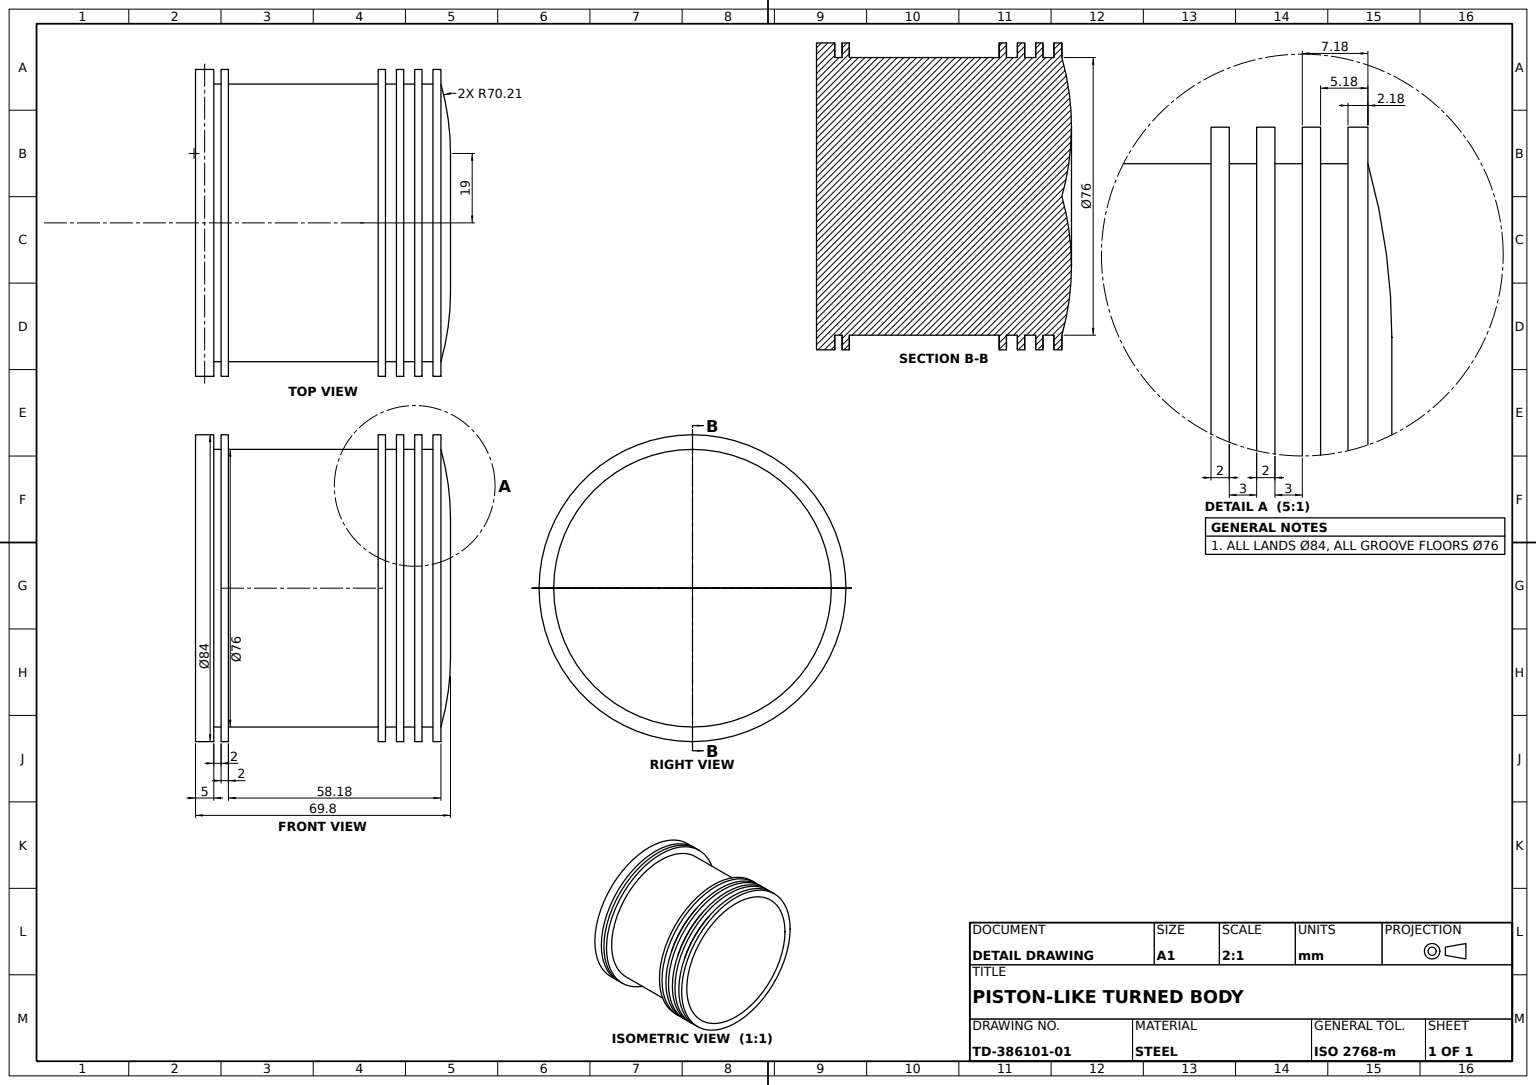
from build123d import *


with BuildPart() as part:
    # Piston Profile Sketch → Piston Body Revolve (revolve)
    with BuildSketch(Plane.XY, mode=Mode.PRIVATE) as piston_body_revolve_sk:
        with BuildLine():
            Line((0, 0), (37, 0))
            Line((37, 0), (42, 0))
            Line((42, 0), (42, 5))
            Line((42, 5), (38, 5))
            Line((38, 5), (38, 7))
            Line((38, 7), (42, 7))
            Line((42, 7), (42, 9))
            Line((42, 9), (38, 9))
            Line((38, 9), (38, 50))
            Line((38, 50), (42, 50))
            Line((42, 50), (42, 52))
            Line((42, 52), (38, 52))
            Line((38, 52), (38, 55))
            Line((38, 55), (42, 55))
            Line((42, 55), (42, 57))
            Line((42, 57), (38, 57))
            Line((38, 57), (38, 60))
            Line((38, 60), (42, 60))
            Line((42, 60), (42, 62))
            Line((42, 62), (38, 62))
            Line((38, 62), (38, 65))
            Line((38, 65), (42, 65))
            Line((42, 65), (42, 67.182193635))
            Line((42, 67.182193635), (38, 67.182193635))
            ThreePointArc((38, 67.182193635), (19, 69.801945586), (0, 67.182193635))
            Line((0, 67.182193635), (0, 0))
        make_face()
    revolve(piston_body_revolve_sk.sketch.rotate(Axis((0, 0, 0), (0, 1, 0)), 90), axis=Axis((0, 0, 0), (0, 1, 0)))


solid = part.part
